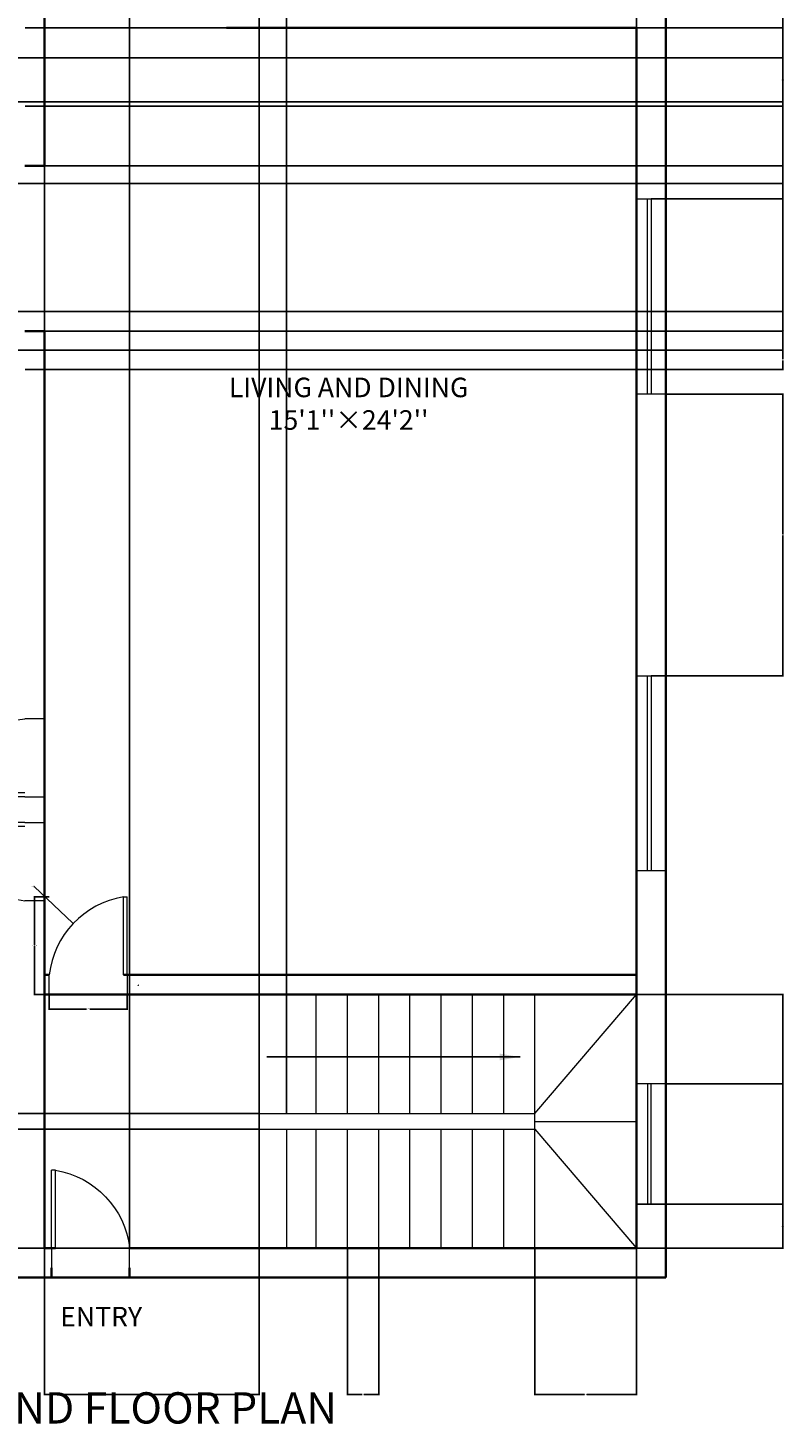
# Model space of a CAD drawing. Units: inches. Extents: x 1108 to 1543, y 442 to 1097.
# Tile 2 of 3: x 1310 to 1543, y 442 to 871. Entities that reach past the tile are written whole.
import ezdxf

# ---------------------------------------------------------------- set-up
doc = ezdxf.new("R2010")
doc.units = ezdxf.units.IN
for name, color, linetype, lineweight in [('A-ANNO-DIMS', 2, 'Continuous', 18), ('A-ANNO-TEXT', 7, 'Continuous', 25), ('A-AREA-IDEN', 7, 'Continuous', 18), ('A-DOOR', 4, 'Continuous', 18), ('A-FLOR-STRS', 7, 'Continuous', 18), ('A-GLAZ', 5, 'Continuous', 18), ('A-WALL', 7, 'Continuous', 35)]:
    doc.layers.add(name, color=color, linetype=linetype, lineweight=lineweight)
doc.styles.get("Standard").update_dxf_attribs({"font": 'times.ttf'})
doc.dimstyles.new('ISO-25', dxfattribs={"dimscale": 2.5, "dimtxt": 2.5, "dimasz": 2.5, "dimexe": 1.25, "dimexo": 0.625, "dimtad": 1, "dimdsep": 46, "dimlunit": 3, "dimtxsty": 'Standard', "dimcen": 2.5, "dimadec": 0, "dimazin": 0, "dimtfac": 1, "dimtmove": 0, "dimatfit": 3, "dimfxl": 1, "dimarcsym": 0})
doc.dimstyles.get("Standard").update_dxf_attribs({"dimtxt": 0.18, "dimasz": 0.18, "dimexe": 0.18, "dimexo": 0.0625, "dimgap": 0.09, "dimtad": 0, "dimtih": 1, "dimtoh": 1, "dimdec": 4, "dimzin": 0, "dimdsep": 46, "dimtxsty": 'Standard', "dimcen": 0.09, "dimadec": 0, "dimazin": 0, "dimtfac": 1, "dimtdec": 4, "dimtofl": 0, "dimtmove": 0, "dimatfit": 3, "dimfxl": 1, "dimtolj": 1, "dimtzin": 0, "dimarcsym": 0})

# ---------------------------------------------------------------- blocks, each defined once
blk = doc.blocks.new('d')
for p, q in [((1309.33, 626.48), (1285.33, 626.48)), ((1285.33, 625.28), (1285.33, 626.48)), ((1309.33, 626.48), (1315.33, 626.48)), ((1309.33, 625.28), (1285.33, 625.28)), ((1315.33, 602.48), (1309.33, 602.48))]:
    blk.add_line(p, q)
blk.add_arc((1312.52, 629.86), 27.57, 189.5705, 263.3671)
blk = doc.blocks.new('WIN-60IN')
for p, q in [((-9, -60), (-9, 0)), ((-9, 0), (0, 0)), ((-5.7, -60), (-5.7, 0)), ((0, 0), (-4.5, 0)), ((-4.5, 0), (-4.5, -60)), ((0, 0), (0, -60)), ((0, -60), (-9, -60)), ((-4.5, -60), (-5.7, -60))]:
    blk.add_line(p, q)
blk = doc.blocks.new('*D9')
at = {"layer": 'A-ANNO-DIMS', "color": 0, "lineweight": -2, "transparency": 16777216}
for p, q in [((1316.74, 603.68), (1312.12, 603.68)), ((1312.3, 603.5), (1312.3, 588.86)), ((1312.3, 573.86), (1312.3, 588.5)), ((1316.74, 573.68), (1312.12, 573.68))]:
    blk.add_line(p, q, dxfattribs=at)
at = {"layer": 'A-ANNO-DIMS', "color": 0, "transparency": 16777216}
for points in [[(1312.27, 603.5), (1312.33, 603.5), (1312.3, 603.68)], [(1312.27, 573.86), (1312.33, 573.86), (1312.3, 573.68)]]:
    blk.add_solid(points, dxfattribs=at)
at = {"layer": 'Defpoints', "color": 0, "transparency": 16777216}
for p in [(1316.8, 603.68), (1312.3, 573.68), (1316.8, 573.68)]:
    blk.add_point(p, dxfattribs=at)
at = {"layer": 'A-ANNO-DIMS', "color": 0, "transparency": 16777216, "insert": (1312.3, 588.68), "char_height": 0.18, "attachment_point": 5}
blk.add_mtext('\\A1;DOOR 30 TYP.', dxfattribs=at)
blk = doc.blocks.new('*D10')
at = {"layer": 'A-ANNO-DIMS', "color": 0, "lineweight": -2, "transparency": 16777216}
for p, q in [((1316.8, 573.62), (1316.8, 569)), ((1340.8, 573.62), (1340.8, 569)), ((1316.98, 569.18), (1328.27, 569.18)), ((1340.62, 569.18), (1329.33, 569.18))]:
    blk.add_line(p, q, dxfattribs=at)
at = {"layer": 'A-ANNO-DIMS', "color": 0, "transparency": 16777216}
for points in [[(1316.98, 569.21), (1316.98, 569.15), (1316.8, 569.18)], [(1340.62, 569.21), (1340.62, 569.15), (1340.8, 569.18)]]:
    blk.add_solid(points, dxfattribs=at)
at = {"layer": 'Defpoints', "color": 0, "transparency": 16777216}
for p in [(1316.8, 573.68), (1340.8, 573.68), (1340.8, 569.18)]:
    blk.add_point(p, dxfattribs=at)
at = {"layer": 'A-ANNO-DIMS', "color": 0, "transparency": 16777216, "insert": (1328.8, 569.18), "char_height": 0.18, "attachment_point": 5}
blk.add_mtext('\\A1;24 TYP.', dxfattribs=at)
blk = doc.blocks.new('*D21')
at = {"layer": 'A-ANNO-DIMS', "color": 0, "lineweight": -2, "transparency": 16777216}
for p, q in [((1506.4, 918.47), (1542.46, 918.47)), ((1542.28, 918.29), (1542.28, 868.51)), ((1542.28, 818.36), (1542.28, 868.14)), ((1506.4, 818.18), (1542.46, 818.18))]:
    blk.add_line(p, q, dxfattribs=at)
at = {"layer": 'A-ANNO-DIMS', "color": 0, "transparency": 16777216}
for points in [[(1542.25, 918.29), (1542.31, 918.29), (1542.28, 918.47)], [(1542.25, 818.36), (1542.31, 818.36), (1542.28, 818.18)]]:
    blk.add_solid(points, dxfattribs=at)
at = {"layer": 'Defpoints', "color": 0, "transparency": 16777216}
for p in [(1506.33, 918.47), (1506.33, 818.18), (1542.28, 818.18)]:
    blk.add_point(p, dxfattribs=at)
at = {"layer": 'A-ANNO-DIMS', "color": 0, "transparency": 16777216, "insert": (1542.28, 868.33), "char_height": 0.18, "attachment_point": 5}
blk.add_mtext('\\A1;100.3', dxfattribs=at)
blk = doc.blocks.new('*D22')
at = {"layer": 'A-ANNO-DIMS', "color": 0, "lineweight": -2, "transparency": 16777216}
for p, q in [((1506.4, 758.18), (1542.46, 758.18)), ((1542.28, 758), (1542.28, 715.08)), ((1542.28, 671.8), (1542.28, 714.72)), ((1506.4, 671.62), (1542.46, 671.62))]:
    blk.add_line(p, q, dxfattribs=at)
at = {"layer": 'A-ANNO-DIMS', "color": 0, "transparency": 16777216}
for points in [[(1542.25, 758), (1542.31, 758), (1542.28, 758.18)], [(1542.25, 671.8), (1542.31, 671.8), (1542.28, 671.62)]]:
    blk.add_solid(points, dxfattribs=at)
at = {"layer": 'Defpoints', "color": 0, "transparency": 16777216}
for p in [(1506.33, 758.18), (1506.33, 671.62), (1542.28, 671.62)]:
    blk.add_point(p, dxfattribs=at)
at = {"layer": 'A-ANNO-DIMS', "color": 0, "transparency": 16777216, "insert": (1542.28, 714.9), "char_height": 0.18, "attachment_point": 5}
blk.add_mtext('\\A1;86.56', dxfattribs=at)
blk = doc.blocks.new('*D23')
at = {"layer": 'A-ANNO-DIMS', "color": 0, "lineweight": -2, "transparency": 16777216}
for p, q in [((1497.4, 509.23), (1542.46, 509.23)), ((1542.28, 509.05), (1542.28, 502.63)), ((1542.28, 495.86), (1542.28, 502.27)), ((1497.4, 495.68), (1542.46, 495.68))]:
    blk.add_line(p, q, dxfattribs=at)
at = {"layer": 'A-ANNO-DIMS', "color": 0, "transparency": 16777216}
for points in [[(1542.25, 509.05), (1542.31, 509.05), (1542.28, 509.23)], [(1542.25, 495.86), (1542.31, 495.86), (1542.28, 495.68)]]:
    blk.add_solid(points, dxfattribs=at)
at = {"layer": 'Defpoints', "color": 0, "transparency": 16777216}
for p in [(1497.33, 509.23), (1542.28, 509.23), (1497.33, 495.68)]:
    blk.add_point(p, dxfattribs=at)
at = {"layer": 'A-ANNO-DIMS', "color": 0, "transparency": 16777216, "insert": (1542.28, 502.45), "char_height": 0.18, "attachment_point": 5}
blk.add_mtext('\\A1;13.547', dxfattribs=at)
blk = doc.blocks.new('*D24')
at = {"layer": 'A-ANNO-DIMS', "color": 0, "lineweight": -2, "transparency": 16777216}
for p, q in [((1506.4, 546.18), (1542.46, 546.18)), ((1542.28, 546), (1542.28, 527.89)), ((1542.28, 509.41), (1542.28, 527.52)), ((1506.4, 509.23), (1542.46, 509.23))]:
    blk.add_line(p, q, dxfattribs=at)
at = {"layer": 'A-ANNO-DIMS', "color": 0, "transparency": 16777216}
for points in [[(1542.25, 546), (1542.31, 546), (1542.28, 546.18)], [(1542.25, 509.41), (1542.31, 509.41), (1542.28, 509.23)]]:
    blk.add_solid(points, dxfattribs=at)
at = {"layer": 'Defpoints', "color": 0, "transparency": 16777216}
for p in [(1506.33, 546.18), (1506.33, 509.23), (1542.28, 509.23)]:
    blk.add_point(p, dxfattribs=at)
at = {"layer": 'A-ANNO-DIMS', "color": 0, "transparency": 16777216, "insert": (1542.28, 527.71), "char_height": 0.18, "attachment_point": 5}
blk.add_mtext('\\A1;36.96', dxfattribs=at)
blk = doc.blocks.new('*D26')
at = {"layer": 'A-ANNO-DIMS', "color": 0, "lineweight": -2, "transparency": 16777216}
for p, q in [((1341.52, 495.74), (1341.52, 1097.43)), ((1341.7, 1097.25), (1361.06, 1097.25)), ((1381.15, 1097.25), (1361.8, 1097.25)), ((1381.33, 495.74), (1381.33, 1097.43))]:
    blk.add_line(p, q, dxfattribs=at)
at = {"layer": 'A-ANNO-DIMS', "color": 0, "transparency": 16777216}
for points in [[(1341.7, 1097.28), (1341.7, 1097.22), (1341.52, 1097.25)], [(1381.15, 1097.28), (1381.15, 1097.22), (1381.33, 1097.25)]]:
    blk.add_solid(points, dxfattribs=at)
at = {"layer": 'Defpoints', "color": 0, "transparency": 16777216}
for p in [(1381.33, 1097.25), (1341.52, 495.68), (1381.33, 495.68)]:
    blk.add_point(p, dxfattribs=at)
at = {"layer": 'A-ANNO-DIMS', "color": 0, "transparency": 16777216, "insert": (1361.43, 1097.25), "char_height": 0.18, "attachment_point": 5}
blk.add_mtext('\\A1;39.81', dxfattribs=at)
blk = doc.blocks.new('*D32')
at = {"layer": 'A-ANNO-DIMS', "color": 0, "lineweight": -2, "transparency": 16777216}
for p, q in [((1315.33, 495.62), (1315.33, 450.55)), ((1381.33, 495.62), (1381.33, 450.55)), ((1315.51, 450.73), (1348.12, 450.73)), ((1381.15, 450.73), (1348.55, 450.73))]:
    blk.add_line(p, q, dxfattribs=at)
at = {"layer": 'A-ANNO-DIMS', "color": 0, "transparency": 16777216}
for points in [[(1315.51, 450.76), (1315.51, 450.7), (1315.33, 450.73)], [(1381.15, 450.76), (1381.15, 450.7), (1381.33, 450.73)]]:
    blk.add_solid(points, dxfattribs=at)
at = {"layer": 'Defpoints', "color": 0, "transparency": 16777216}
for p in [(1315.33, 495.68), (1381.33, 495.68), (1381.33, 450.73)]:
    blk.add_point(p, dxfattribs=at)
at = {"layer": 'A-ANNO-DIMS', "color": 0, "transparency": 16777216, "insert": (1348.33, 450.73), "char_height": 0.18, "attachment_point": 5}
blk.add_mtext('\\A1;66', dxfattribs=at)
blk = doc.blocks.new('*D33')
at = {"layer": 'A-ANNO-DIMS', "color": 0, "lineweight": -2, "transparency": 16777216}
for p, q in [((1497.4, 573.68), (1542.46, 573.68)), ((1542.28, 573.5), (1542.28, 534.86)), ((1542.28, 495.86), (1542.28, 534.5)), ((1497.4, 495.68), (1542.46, 495.68))]:
    blk.add_line(p, q, dxfattribs=at)
at = {"layer": 'A-ANNO-DIMS', "color": 0, "transparency": 16777216}
for points in [[(1542.25, 573.5), (1542.31, 573.5), (1542.28, 573.68)], [(1542.25, 495.86), (1542.31, 495.86), (1542.28, 495.68)]]:
    blk.add_solid(points, dxfattribs=at)
at = {"layer": 'Defpoints', "color": 0, "transparency": 16777216}
for p in [(1497.33, 573.68), (1542.28, 573.68), (1497.33, 495.68)]:
    blk.add_point(p, dxfattribs=at)
at = {"layer": 'A-ANNO-DIMS', "color": 0, "transparency": 16777216, "insert": (1542.28, 534.68), "char_height": 0.18, "attachment_point": 5}
blk.add_mtext('\\A1;78', dxfattribs=at)
blk = doc.blocks.new('*D34')
at = {"layer": 'A-ANNO-DIMS', "color": 0, "lineweight": -2, "transparency": 16777216}
for p, q in [((1466.07, 495.62), (1466.07, 450.55)), ((1497.33, 495.62), (1497.33, 450.55)), ((1466.25, 450.73), (1481.33, 450.73)), ((1497.15, 450.73), (1482.08, 450.73))]:
    blk.add_line(p, q, dxfattribs=at)
at = {"layer": 'A-ANNO-DIMS', "color": 0, "transparency": 16777216}
for points in [[(1466.25, 450.76), (1466.25, 450.7), (1466.07, 450.73)], [(1497.15, 450.76), (1497.15, 450.7), (1497.33, 450.73)]]:
    blk.add_solid(points, dxfattribs=at)
at = {"layer": 'Defpoints', "color": 0, "transparency": 16777216}
for p in [(1466.07, 495.68), (1497.33, 495.68), (1497.33, 450.73)]:
    blk.add_point(p, dxfattribs=at)
at = {"layer": 'A-ANNO-DIMS', "color": 0, "transparency": 16777216, "insert": (1481.7, 450.73), "char_height": 0.18, "attachment_point": 5}
blk.add_mtext('\\A1;31.26', dxfattribs=at)
blk = doc.blocks.new('*D35')
at = {"layer": 'A-ANNO-DIMS', "color": 0, "lineweight": -2, "transparency": 16777216}
for p, q in [((1408.47, 495.62), (1408.47, 450.55)), ((1418.07, 495.62), (1418.07, 450.55)), ((1408.65, 450.73), (1413.03, 450.73)), ((1417.89, 450.73), (1413.52, 450.73))]:
    blk.add_line(p, q, dxfattribs=at)
at = {"layer": 'A-ANNO-DIMS', "color": 0, "transparency": 16777216}
for points in [[(1408.65, 450.76), (1408.65, 450.7), (1408.47, 450.73)], [(1417.89, 450.76), (1417.89, 450.7), (1418.07, 450.73)]]:
    blk.add_solid(points, dxfattribs=at)
at = {"layer": 'Defpoints', "color": 0, "transparency": 16777216}
for p in [(1408.47, 495.68), (1418.07, 495.68), (1418.07, 450.73)]:
    blk.add_point(p, dxfattribs=at)
at = {"layer": 'A-ANNO-DIMS', "color": 0, "transparency": 16777216, "insert": (1413.27, 450.73), "char_height": 0.18, "attachment_point": 5}
blk.add_mtext('\\A1;9.6', dxfattribs=at)
blk = doc.blocks.new('*D36')
at = {"layer": 'A-ANNO-DIMS', "color": 0, "lineweight": -2, "transparency": 16777216}
for p, q in [((1381.27, 532.28), (1108.2, 532.28)), ((1108.38, 532.1), (1108.38, 514.16)), ((1108.38, 495.86), (1108.38, 513.8)), ((1381.27, 495.68), (1108.2, 495.68))]:
    blk.add_line(p, q, dxfattribs=at)
at = {"layer": 'A-ANNO-DIMS', "color": 0, "transparency": 16777216}
for points in [[(1108.35, 532.1), (1108.41, 532.1), (1108.38, 532.28)], [(1108.35, 495.86), (1108.41, 495.86), (1108.38, 495.68)]]:
    blk.add_solid(points, dxfattribs=at)
at = {"layer": 'Defpoints', "color": 0, "transparency": 16777216}
for p in [(1381.33, 532.28), (1108.38, 495.68), (1381.33, 495.68)]:
    blk.add_point(p, dxfattribs=at)
at = {"layer": 'A-ANNO-DIMS', "color": 0, "transparency": 16777216, "insert": (1108.38, 513.98), "char_height": 0.18, "attachment_point": 5}
blk.add_mtext('\\A1;36.6', dxfattribs=at)
blk = doc.blocks.new('*D37')
at = {"layer": 'A-ANNO-DIMS', "color": 0, "lineweight": -2, "transparency": 16777216}
for p, q in [((1309.4, 771.68), (1542.46, 771.68)), ((1542.28, 771.5), (1542.28, 768.86)), ((1542.28, 765.86), (1542.28, 768.5)), ((1309.4, 765.68), (1542.46, 765.68))]:
    blk.add_line(p, q, dxfattribs=at)
at = {"layer": 'A-ANNO-DIMS', "color": 0, "transparency": 16777216}
for points in [[(1542.25, 771.5), (1542.31, 771.5), (1542.28, 771.68)], [(1542.25, 765.86), (1542.31, 765.86), (1542.28, 765.68)]]:
    blk.add_solid(points, dxfattribs=at)
at = {"layer": 'Defpoints', "color": 0, "transparency": 16777216}
for p in [(1309.33, 771.68), (1542.28, 771.68), (1309.33, 765.68)]:
    blk.add_point(p, dxfattribs=at)
at = {"layer": 'A-ANNO-DIMS', "color": 0, "transparency": 16777216, "insert": (1542.28, 768.68), "char_height": 0.18, "attachment_point": 5}
blk.add_mtext('\\A1;6', dxfattribs=at)
blk = doc.blocks.new('*D39')
at = {"layer": 'A-ANNO-DIMS', "color": 0, "lineweight": -2, "transparency": 16777216}
for p, q in [((1315.4, 828.29), (1542.46, 828.29)), ((1542.28, 828.11), (1542.28, 803.07)), ((1542.28, 777.66), (1542.28, 802.7)), ((1315.4, 777.48), (1542.46, 777.48))]:
    blk.add_line(p, q, dxfattribs=at)
at = {"layer": 'A-ANNO-DIMS', "color": 0, "transparency": 16777216}
for points in [[(1542.25, 828.11), (1542.31, 828.11), (1542.28, 828.29)], [(1542.25, 777.66), (1542.31, 777.66), (1542.28, 777.48)]]:
    blk.add_solid(points, dxfattribs=at)
at = {"layer": 'Defpoints', "color": 0, "transparency": 16777216}
for p in [(1315.33, 828.29), (1542.28, 828.29), (1315.33, 777.48)]:
    blk.add_point(p, dxfattribs=at)
at = {"layer": 'A-ANNO-DIMS', "color": 0, "transparency": 16777216, "insert": (1542.28, 802.88), "char_height": 0.18, "attachment_point": 5}
blk.add_mtext('\\A1;50.81', dxfattribs=at)
blk = doc.blocks.new('*D42')
at = {"layer": 'A-ANNO-DIMS', "color": 0, "lineweight": -2, "transparency": 16777216}
for p, q in [((1175.72, 822.87), (1542.46, 822.87)), ((1542.28, 822.69), (1542.28, 803.38)), ((1542.28, 783.72), (1542.28, 803.02)), ((1175.72, 783.54), (1542.46, 783.54))]:
    blk.add_line(p, q, dxfattribs=at)
at = {"layer": 'A-ANNO-DIMS', "color": 0, "transparency": 16777216}
for points in [[(1542.25, 822.69), (1542.31, 822.69), (1542.28, 822.87)], [(1542.25, 783.72), (1542.31, 783.72), (1542.28, 783.54)]]:
    blk.add_solid(points, dxfattribs=at)
at = {"layer": 'Defpoints', "color": 0, "transparency": 16777216}
for p in [(1175.65, 822.87), (1542.28, 822.87), (1175.65, 783.54)]:
    blk.add_point(p, dxfattribs=at)
at = {"layer": 'A-ANNO-DIMS', "color": 0, "transparency": 16777216, "insert": (1542.28, 803.2), "char_height": 0.18, "attachment_point": 5}
blk.add_mtext('\\A1;39.33', dxfattribs=at)
blk = doc.blocks.new('*D43')
at = {"layer": 'A-ANNO-DIMS', "color": 0, "lineweight": -2, "transparency": 16777216}
for p, q in [((1175.72, 783.54), (1542.46, 783.54)), ((1542.28, 783.36), (1542.28, 777.79)), ((1542.28, 771.86), (1542.28, 777.43)), ((1177.4, 771.68), (1542.46, 771.68))]:
    blk.add_line(p, q, dxfattribs=at)
at = {"layer": 'A-ANNO-DIMS', "color": 0, "transparency": 16777216}
for points in [[(1542.25, 783.36), (1542.31, 783.36), (1542.28, 783.54)], [(1542.25, 771.86), (1542.31, 771.86), (1542.28, 771.68)]]:
    blk.add_solid(points, dxfattribs=at)
at = {"layer": 'Defpoints', "color": 0, "transparency": 16777216}
for p in [(1175.65, 783.54), (1177.33, 771.68), (1542.28, 771.68)]:
    blk.add_point(p, dxfattribs=at)
at = {"layer": 'A-ANNO-DIMS', "color": 0, "transparency": 16777216, "insert": (1542.28, 777.61), "char_height": 0.18, "attachment_point": 5}
blk.add_mtext('\\A1;11.857', dxfattribs=at)
blk = doc.blocks.new('*D46')
at = {"layer": 'A-ANNO-DIMS', "color": 0, "lineweight": -2, "transparency": 16777216}
for p, q in [((1309.397156, 870.679098), (1542.464656, 870.679098)), ((1542.284656, 870.499098), (1542.284656, 858.859098)), ((1542.284656, 846.859098), (1542.284656, 858.499098)), ((1309.397156, 846.679098), (1542.464656, 846.679098))]:
    blk.add_line(p, q, dxfattribs=at)
at = {"layer": 'A-ANNO-DIMS', "color": 0, "transparency": 16777216}
for points in [[(1542.254656, 870.499098), (1542.314656, 870.499098), (1542.284656, 870.679098)], [(1542.254656, 846.859098), (1542.314656, 846.859098), (1542.284656, 846.679098)]]:
    blk.add_solid(points, dxfattribs=at)
at = {"layer": 'Defpoints', "color": 0, "transparency": 16777216}
for p in [(1309.334656, 870.679098), (1542.284656, 870.679098), (1309.334656, 846.679098)]:
    blk.add_point(p, dxfattribs=at)
at = {"layer": 'A-ANNO-DIMS', "color": 0, "transparency": 16777216, "insert": (1542.284656, 858.679098), "char_height": 0.18, "attachment_point": 5}
blk.add_mtext('\\A1;24', dxfattribs=at)
blk = doc.blocks.new('*D47')
at = {"layer": 'A-ANNO-DIMS', "color": 0, "lineweight": -2, "transparency": 16777216}
for p, q in [((1309.4, 846.68), (1542.46, 846.68)), ((1542.28, 846.5), (1542.28, 837.67)), ((1542.28, 828.47), (1542.28, 837.3)), ((1309.4, 828.29), (1542.46, 828.29))]:
    blk.add_line(p, q, dxfattribs=at)
at = {"layer": 'A-ANNO-DIMS', "color": 0, "transparency": 16777216}
for points in [[(1542.25, 846.5), (1542.31, 846.5), (1542.28, 846.68)], [(1542.25, 828.47), (1542.31, 828.47), (1542.28, 828.29)]]:
    blk.add_solid(points, dxfattribs=at)
at = {"layer": 'Defpoints', "color": 0, "transparency": 16777216}
for p in [(1309.33, 846.68), (1542.28, 846.68), (1309.33, 828.29)]:
    blk.add_point(p, dxfattribs=at)
at = {"layer": 'A-ANNO-DIMS', "color": 0, "transparency": 16777216, "insert": (1542.28, 837.48), "char_height": 0.18, "attachment_point": 5}
blk.add_mtext('\\A1;18.39', dxfattribs=at)
blk = doc.blocks.new('*D48')
at = {"layer": 'A-ANNO-DIMS', "color": 0, "lineweight": -2, "transparency": 16777216}
for p, q in [((1267.67, 861.48), (1542.46, 861.48)), ((1542.28, 861.3), (1542.28, 854.89)), ((1542.28, 848.11), (1542.28, 854.52)), ((1269.67, 847.93), (1542.46, 847.93))]:
    blk.add_line(p, q, dxfattribs=at)
at = {"layer": 'A-ANNO-DIMS', "color": 0, "transparency": 16777216}
for points in [[(1542.25, 861.3), (1542.31, 861.3), (1542.28, 861.48)], [(1542.25, 848.11), (1542.31, 848.11), (1542.28, 847.93)]]:
    blk.add_solid(points, dxfattribs=at)
at = {"layer": 'Defpoints', "color": 0, "transparency": 16777216}
for p in [(1267.61, 861.48), (1542.28, 861.48), (1269.61, 847.93)]:
    blk.add_point(p, dxfattribs=at)
at = {"layer": 'A-ANNO-DIMS', "color": 0, "transparency": 16777216, "insert": (1542.28, 854.71), "char_height": 0.18, "attachment_point": 5}
blk.add_mtext('\\A1;13.556', dxfattribs=at)
blk = doc.blocks.new('*D50')
at = {"layer": 'A-ANNO-DIMS', "color": 0, "lineweight": -2, "transparency": 16777216}
for p, q in [((1381.33, 537.14), (1381.33, 1097.43)), ((1381.51, 1097.25), (1385.16, 1097.25)), ((1389.56, 1097.25), (1385.91, 1097.25)), ((1389.74, 537.14), (1389.74, 1097.43))]:
    blk.add_line(p, q, dxfattribs=at)
at = {"layer": 'A-ANNO-DIMS', "color": 0, "transparency": 16777216}
for points in [[(1381.51, 1097.28), (1381.51, 1097.22), (1381.33, 1097.25)], [(1389.56, 1097.28), (1389.56, 1097.22), (1389.74, 1097.25)]]:
    blk.add_solid(points, dxfattribs=at)
at = {"layer": 'Defpoints', "color": 0, "transparency": 16777216}
for p in [(1389.74, 1097.25), (1381.33, 537.08), (1389.74, 537.08)]:
    blk.add_point(p, dxfattribs=at)
at = {"layer": 'A-ANNO-DIMS', "color": 0, "transparency": 16777216, "insert": (1385.54, 1097.25), "char_height": 0.18, "attachment_point": 5}
blk.add_mtext('\\A1;8.404', dxfattribs=at)
blk = doc.blocks.new('*D51')
at = {"layer": 'A-ANNO-DIMS', "color": 0, "lineweight": -2, "transparency": 16777216}
for p, q in [((1381.27, 537.08), (1108.2, 537.08)), ((1108.38, 536.9), (1108.38, 534.86)), ((1381.27, 532.28), (1108.2, 532.28)), ((1108.38, 532.46), (1108.38, 534.5))]:
    blk.add_line(p, q, dxfattribs=at)
at = {"layer": 'A-ANNO-DIMS', "color": 0, "transparency": 16777216}
for points in [[(1108.35, 536.9), (1108.41, 536.9), (1108.38, 537.08)], [(1108.35, 532.46), (1108.41, 532.46), (1108.38, 532.28)]]:
    blk.add_solid(points, dxfattribs=at)
at = {"layer": 'Defpoints', "color": 0, "transparency": 16777216}
for p in [(1381.33, 537.08), (1108.38, 532.28), (1381.33, 532.28)]:
    blk.add_point(p, dxfattribs=at)
at = {"layer": 'A-ANNO-DIMS', "color": 0, "transparency": 16777216, "insert": (1108.38, 534.68), "char_height": 0.18, "attachment_point": 5}
blk.add_mtext('\\A1;4.8', dxfattribs=at)
blk = doc.blocks.new('*D52')
at = {"layer": 'A-ANNO-DIMS', "color": 0, "lineweight": -2, "transparency": 16777216}
for p, q in [((1315.33, 573.74), (1315.33, 1097.43)), ((1315.51, 1097.25), (1406.07, 1097.25)), ((1497.15, 1097.25), (1406.6, 1097.25)), ((1497.33, 573.74), (1497.33, 1097.43))]:
    blk.add_line(p, q, dxfattribs=at)
at = {"layer": 'A-ANNO-DIMS', "color": 0, "transparency": 16777216}
for points in [[(1315.51, 1097.28), (1315.51, 1097.22), (1315.33, 1097.25)], [(1497.15, 1097.28), (1497.15, 1097.22), (1497.33, 1097.25)]]:
    blk.add_solid(points, dxfattribs=at)
at = {"layer": 'Defpoints', "color": 0, "transparency": 16777216}
for p in [(1497.33, 1097.25), (1315.33, 573.68), (1497.33, 573.68)]:
    blk.add_point(p, dxfattribs=at)
at = {"layer": 'A-ANNO-DIMS', "color": 0, "transparency": 16777216, "insert": (1406.33, 1097.25), "char_height": 0.18, "attachment_point": 5}
blk.add_mtext('\\A1;182', dxfattribs=at)
blk = doc.blocks.new('*D54')
at = {"layer": 'A-ANNO-DIMS', "color": 0, "lineweight": -2, "transparency": 16777216}
for p, q in [((1312.02, 606.87), (1312.2, 606.87)), ((1312.2, 606.87), (1324.07, 595.61)), ((1344.09, 576.49), (1344.27, 576.49)), ((1344.18, 576.4), (1344.18, 576.58))]:
    blk.add_line(p, q, dxfattribs=at)
at = {"layer": 'A-ANNO-DIMS', "color": 0, "transparency": 16777216}
blk.add_solid([(1324.09, 595.63), (1324.05, 595.58), (1324.2, 595.48)], dxfattribs=at)
at = {"layer": 'Defpoints', "color": 0, "transparency": 16777216}
for p in [(1324.2, 595.48), (1344.18, 576.49)]:
    blk.add_point(p, dxfattribs=at)
at = {"layer": 'A-ANNO-DIMS', "color": 0, "transparency": 16777216, "insert": (1311.56, 606.87), "char_height": 0.18, "attachment_point": 5}
blk.add_mtext('\\A1;R27.57', dxfattribs=at)

msp = doc.modelspace()

# ---------------------------------------------------------------- linework, layer by layer
at = {"layer": 'A-DOOR'}
msp.add_line((1315.3347, 626.4791), (1315.3347, 602.4791), dxfattribs=at)
at = {"layer": 'A-FLOR-STRS'}
for p, q in [((1389.7386, 573.6791), (1389.7386, 537.0791)), ((1398.875, 537.0791), (1398.875, 573.6791)), ((1408.475, 537.0791), (1408.475, 573.6791)), ((1418.075, 537.0791), (1418.075, 573.6791)), ((1427.675, 537.0791), (1427.675, 573.6791)), ((1437.275, 537.0791), (1437.275, 573.6791)), ((1446.875, 537.0791), (1446.875, 573.6791)), ((1456.475, 537.0791), (1456.475, 573.6791)), ((1466.075, 495.6791), (1466.075, 573.6791)), ((1466.075, 537.0791), (1497.3347, 573.6791)), ((1381.3347, 495.6791), (1381.3347, 537.0791)), ((1381.3347, 537.0791), (1466.075, 537.0791)), ((1381.3347, 532.2791), (1466.075, 532.2791)), ((1389.7386, 532.2791), (1389.7386, 495.6791)), ((1398.875, 495.6791), (1398.875, 532.2791)), ((1408.475, 495.6791), (1408.475, 532.2791)), ((1418.075, 495.6791), (1418.075, 532.2791)), ((1427.675, 495.6791), (1427.675, 532.2791)), ((1437.275, 495.6791), (1437.275, 532.2791)), ((1446.875, 495.6791), (1446.875, 532.2791)), ((1456.475, 495.6791), (1456.475, 532.2791)), ((1466.075, 534.6791), (1497.3347, 534.6791)), ((1466.075, 532.2791), (1497.3347, 495.6791)), ((1497.3347, 495.6791), (1381.3347, 495.6791))]:
    msp.add_line(p, q, dxfattribs=at)
at = {"layer": 'A-GLAZ'}
for p, q in [((1506.3347, 546.184), (1497.3347, 546.184)), ((1497.3347, 546.184), (1497.3347, 509.2262)), ((1501.8347, 546.184), (1500.6347, 546.184)), ((1500.6347, 546.184), (1500.6347, 509.2262)), ((1501.8347, 509.2262), (1501.8347, 546.184)), ((1506.3347, 510.184), (1506.3347, 546.184)), ((1497.3347, 509.2262), (1506.3347, 509.2262)), ((1506.3347, 509.2262), (1506.3347, 510.184))]:
    msp.add_line(p, q, dxfattribs=at)
at = {"layer": 'A-WALL'}
for p, q in [((1506.3347, 486.6791), (1506.3347, 1029.6791)), ((1315.3347, 918.6791), (1315.3347, 828.2882)), ((1371.3347, 870.6791), (1497.3347, 870.6791)), ((1497.3347, 495.6791), (1497.3347, 870.6791)), ((1309.3347, 828.2882), (1315.3347, 828.2882)), ((1309.3347, 777.4792), (1315.3347, 777.4792)), ((1315.3347, 777.4792), (1315.3347, 495.6791)), ((1316.8007, 579.6791), (1315.3347, 579.6791)), ((1497.3347, 579.6791), (1339.6007, 579.6791)), ((1497.3347, 573.6791), (1315.3347, 573.6791)), ((1318.7247, 495.6791), (1315.3347, 495.6791)), ((1497.3347, 495.6791), (1341.5247, 495.6791)), ((1317.5247, 489.6791), (1317.5247, 486.6791)), ((1341.5247, 489.6791), (1341.5247, 486.6791)), ((1315.3347, 486.6791), (1144.3347, 486.6791)), ((1506.3347, 486.6791), (1315.3347, 486.6791))]:
    msp.add_line(p, q, dxfattribs=at)

# ---------------------------------------------------------------- block references
at = {"layer": 'A-DOOR', "xscale": -1}
for p, rotation in [((0, 1260.8655), 180), ((1944.0038, 1805.0138), 90)]:
    msp.add_blockref('d', p, dxfattribs=dict(at, rotation=rotation))
at = {"layer": 'A-DOOR'}
msp.add_blockref('d', (0, 0), dxfattribs=at)
at = {"layer": 'A-DOOR', "rotation": 270}
msp.add_blockref('d', (714.3216, 1889.0138), dxfattribs=at)
at = {"layer": 'A-GLAZ'}
for p in [(1506.3347, 818.1791), (1506.3347, 671.6176)]:
    msp.add_blockref('WIN-60IN', p, dxfattribs=at)

# ---------------------------------------------------------------- texts
at = {"layer": 'A-ANNO-TEXT', "insert": (1202.8439, 451.4335), "char_height": 9.6, "attachment_point": 1}
msp.add_mtext_dynamic_manual_height_columns('\\pxqc;GROUND FLOOR PLAN', width=269.09847, gutter_width=12.5, heights=[0], dxfattribs=at)
at = {"layer": 'A-AREA-IDEN', "char_height": 6, "attachment_point": 1}
for s, insert in [("\\pxqc;LIVING AND DINING\\P15'1''×24'2''", (1274.2643, 763.2073)), ('\\pxqc;ENTRY', (1198.21, 477.6754))]:
    msp.add_mtext_dynamic_manual_height_columns(s, width=269.09847, gutter_width=12.5, heights=[0], dxfattribs=dict(at, insert=insert))

# ---------------------------------------------------------------- dimensions: what is measured, and where the dimension line sits
at = {"layer": 'A-ANNO-DIMS'}
for base, p1, p2, override, picture, middle in [((1497.3347, 1097.2479), (1315.3347, 573.6791), (1497.3347, 573.6791), {"dimdec": 0, "dimlfac": 1, "dimrnd": 0, "dimzin": 0, "dimdsep": 46, "dimlunit": 2}, '*D52', (1406.3347, 1097.2479)), ((1381.3347, 1097.2479), (1341.5247, 495.6791), (1381.3347, 495.6791), {"dimdec": 2, "dimlfac": 1, "dimrnd": 0, "dimzin": 0, "dimdsep": 46, "dimlunit": 2}, '*D26', (1361.4297, 1097.2479)), ((1389.7386, 1097.2479), (1381.3347, 537.0791), (1389.7386, 537.0791), {"dimdec": 3, "dimlfac": 1, "dimrnd": 0, "dimzin": 0, "dimdsep": 46, "dimlunit": 2}, '*D50', (1385.5366, 1097.2479)), ((1381.3347, 450.7291), (1315.3347, 495.6791), (1381.3347, 495.6791), {"dimdec": 0, "dimlfac": 1, "dimrnd": 0, "dimzin": 0, "dimdsep": 46, "dimlunit": 2}, '*D32', (1348.3347, 450.7291)), ((1418.075, 450.7291), (1408.475, 495.6791), (1418.075, 495.6791), {"dimdec": 1, "dimlfac": 1, "dimrnd": 0, "dimzin": 0, "dimdsep": 46, "dimlunit": 2}, '*D35', (1413.275, 450.7291)), ((1497.3347, 450.7291), (1466.075, 495.6791), (1497.3347, 495.6791), {"dimdec": 2, "dimlfac": 1, "dimrnd": 0, "dimzin": 0, "dimdsep": 46, "dimlunit": 2}, '*D34', (1481.7048, 450.7291))]:
    dim = msp.add_linear_dim(base=base, p1=p1, p2=p2, dimstyle='Standard', override=override, dxfattribs=at)
    dim.commit()
    dim.dimension.update_dxf_attribs({"geometry": picture, "text_midpoint": middle})
for base, p1, p2, override, picture, middle in [((1542.2847, 818.1791), (1506.3347, 918.4725), (1506.3347, 818.1791), {"dimdec": 1, "dimlfac": 1, "dimrnd": 0, "dimzin": 0, "dimdsep": 46, "dimlunit": 2}, '*D21', (1542.2847, 868.3258)), ((1542.2847, 870.6791), (1309.3347, 846.6791), (1309.3347, 870.6791), {"dimdec": 0, "dimlfac": 1, "dimrnd": 0, "dimzin": 0, "dimdsep": 46, "dimlunit": 2}, '*D46', (1542.2847, 858.6791)), ((1542.2847, 861.4845), (1269.6075, 847.9289), (1267.6075, 861.4845), {"dimdec": 3, "dimlfac": 1, "dimrnd": 0, "dimzin": 0, "dimdsep": 46, "dimlunit": 2}, '*D48', (1542.2847, 854.7067)), ((1542.2847, 846.6791), (1309.3347, 828.2882), (1309.3347, 846.6791), {"dimdec": 2, "dimlfac": 1, "dimrnd": 0, "dimzin": 0, "dimdsep": 46, "dimlunit": 2}, '*D47', (1542.2847, 837.4836)), ((1542.2847, 828.2882), (1315.3347, 777.4792), (1315.3347, 828.2882), {"dimdec": 2, "dimlfac": 1, "dimrnd": 0, "dimzin": 0, "dimdsep": 46, "dimlunit": 2}, '*D39', (1542.2847, 802.8837)), ((1542.2847, 822.8655), (1175.6532, 783.5357), (1175.6532, 822.8655), {"dimdec": 2, "dimlfac": 1, "dimrnd": 0, "dimzin": 0, "dimdsep": 46, "dimlunit": 2}, '*D42', (1542.2847, 803.2006)), ((1542.2847, 771.6791), (1175.6532, 783.5357), (1177.3347, 771.6791), {"dimdec": 3, "dimlfac": 1, "dimrnd": 0, "dimzin": 0, "dimdsep": 46, "dimlunit": 2}, '*D43', (1542.2847, 777.6074)), ((1542.2847, 771.6791), (1309.3347, 765.6791), (1309.3347, 771.6791), {"dimdec": 0, "dimlfac": 1, "dimrnd": 0, "dimzin": 0, "dimdsep": 46, "dimlunit": 2}, '*D37', (1542.2847, 768.6791)), ((1542.2847, 671.6176), (1506.3347, 758.1791), (1506.3347, 671.6176), {"dimdec": 2, "dimlfac": 1, "dimrnd": 0, "dimzin": 0, "dimdsep": 46, "dimlunit": 2}, '*D22', (1542.2847, 714.8984)), ((1542.2847, 573.6791), (1497.3347, 495.6791), (1497.3347, 573.6791), {"dimdec": 0, "dimlfac": 1, "dimrnd": 0, "dimzin": 0, "dimdsep": 46, "dimlunit": 2}, '*D33', (1542.2847, 534.6791)), ((1542.2847, 509.2262), (1506.3347, 546.184), (1506.3347, 509.2262), {"dimdec": 2, "dimlfac": 1, "dimrnd": 0, "dimzin": 0, "dimdsep": 46, "dimlunit": 2}, '*D24', (1542.2847, 527.7051)), ((1108.3847, 532.2791), (1381.3347, 537.0791), (1381.3347, 532.2791), {"dimdec": 1, "dimlfac": 1, "dimrnd": 0, "dimzin": 0, "dimdsep": 46, "dimlunit": 2}, '*D51', (1108.3847, 534.6791)), ((1108.3847, 495.6791), (1381.3347, 532.2791), (1381.3347, 495.6791), {"dimdec": 1, "dimlfac": 1, "dimrnd": 0, "dimzin": 0, "dimdsep": 46, "dimlunit": 2}, '*D36', (1108.3847, 513.9791)), ((1542.2847, 509.2262), (1497.3347, 495.6791), (1497.3347, 509.2262), {"dimdec": 3, "dimlfac": 1, "dimrnd": 0, "dimzin": 0, "dimdsep": 46, "dimlunit": 2}, '*D23', (1542.2847, 502.4527))]:
    dim = msp.add_linear_dim(base=base, p1=p1, p2=p2, angle=90, dimstyle='Standard', override=override, dxfattribs=at)
    dim.commit()
    dim.dimension.update_dxf_attribs({"geometry": picture, "text_midpoint": middle})
dim = msp.add_radius_dim(center=(1344.1842, 576.4948), mpoint=(1324.1971, 595.4819), dimstyle='Standard', override={"dimdec": 2, "dimlfac": 1, "dimrnd": 0, "dimzin": 0, "dimdsep": 46, "dimlunit": 2}, dxfattribs=at)
dim.commit()
dim.dimension.update_dxf_attribs({"geometry": '*D54', "text_midpoint": (1311.5554, 606.8742), "dimtype": 164})
dim = msp.add_linear_dim(base=(1312.3007, 573.6791), p1=(1316.8007, 603.6791), p2=(1316.8007, 573.6791), angle=270, text='DOOR <> TYP.', dimstyle='Standard', override={"dimdec": 0, "dimlfac": 1, "dimrnd": 0, "dimzin": 0, "dimdsep": 46, "dimlunit": 2}, dxfattribs=at)
dim.commit()
dim.dimension.update_dxf_attribs({"geometry": '*D9', "text_midpoint": (1312.3007, 588.6791)})
dim = msp.add_linear_dim(base=(1340.8007, 569.1791), p1=(1316.8007, 573.6791), p2=(1340.8007, 573.6791), text='<> TYP.', dimstyle='Standard', override={"dimdec": 0, "dimlfac": 1, "dimrnd": 0, "dimzin": 0, "dimdsep": 46, "dimlunit": 2}, dxfattribs=at)
dim.commit()
dim.dimension.update_dxf_attribs({"geometry": '*D10', "text_midpoint": (1328.8007, 569.1791)})

# ---------------------------------------------------------------- leaders
at = {"layer": 'A-FLOR-STRS'}
msp.add_leader([(1461.496, 554.4672), (1383.6896, 554.4672)], dimstyle='ISO-25', dxfattribs=at)

doc.saveas('drawing.dxf')
